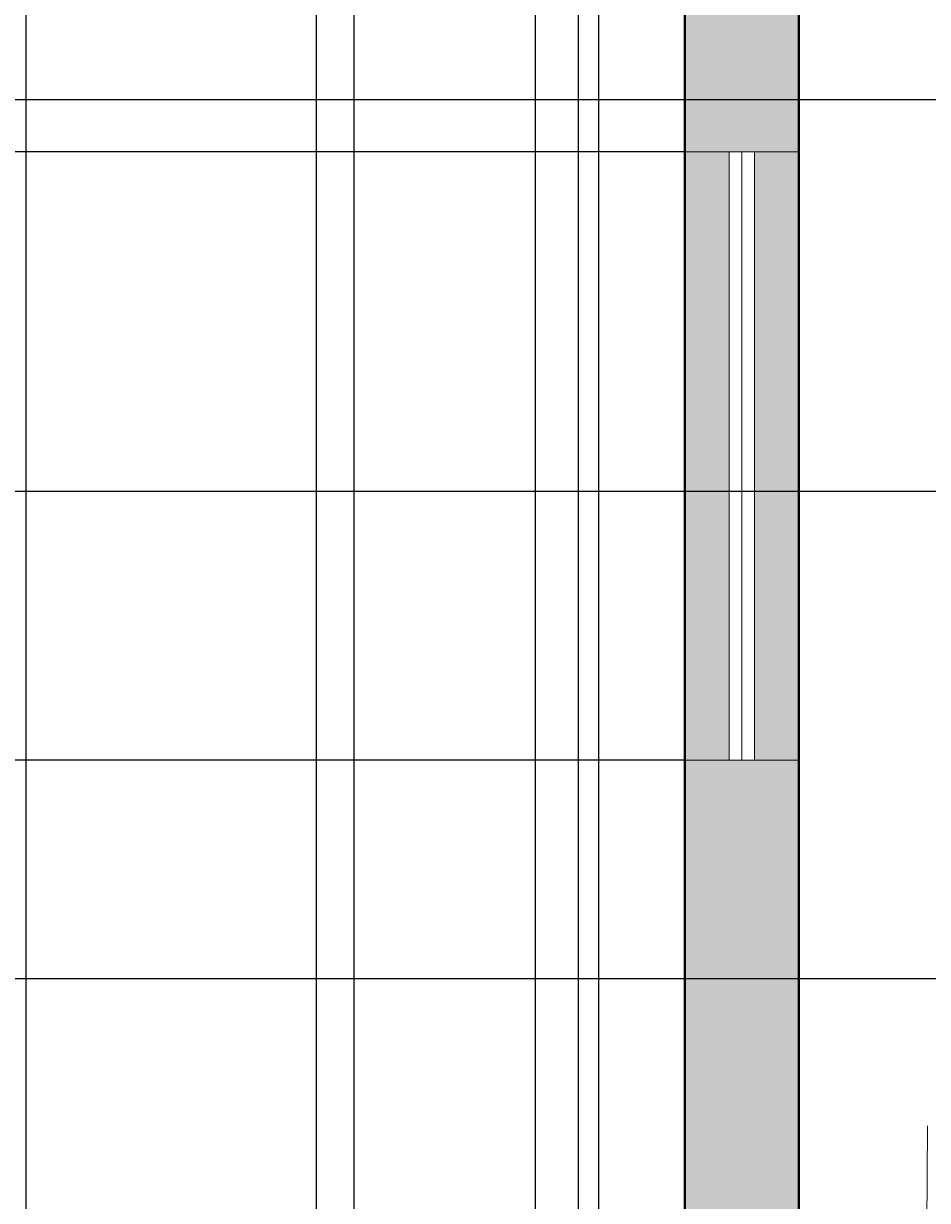
# Model space of a CAD drawing. Units: inches. Extents: x 818 to 1898, y 976 to 2364.
# Tile 33 of 96: x 1207 to 1278, y 1780 to 1873. Entities that reach past the tile are written whole.
import ezdxf

# ---------------------------------------------------------------- set-up
doc = ezdxf.new("R2010")
doc.units = ezdxf.units.IN
doc.header["$LTSCALE"] = 5
doc.header["$MEASUREMENT"] = 0
for name, color, linetype, lineweight in [('A-ANNO-DIMS', 2, 'Continuous', 18), ('A-FURN', 8, 'Continuous', 18), ('A-GLAZ', 4, 'Continuous', 18), ('A-WALL', 7, 'Continuous', 40)]:
    doc.layers.add(name, color=color, linetype=linetype, lineweight=lineweight)
doc.layers.add('A-GLAZ-PATT', color=141, linetype='Continuous', lineweight=9, true_color=0xadddf7)
doc.layers.add('A-WALL-PATT', color=251, linetype='Continuous', lineweight=13, true_color=0x636466)
doc.styles.get("Standard").update_dxf_attribs({"font": 'arial.ttf'})
doc.dimstyles.get("Standard").update_dxf_attribs({"dimtxt": 0.18, "dimasz": 0.18, "dimexe": 0.18, "dimexo": 0.0625, "dimgap": 0.09, "dimtad": 0, "dimtih": 1, "dimtoh": 1, "dimdec": 4, "dimzin": 0, "dimdsep": 46, "dimtxsty": 'Standard', "dimcen": 0.09, "dimadec": 0, "dimazin": 0, "dimtfac": 1, "dimtdec": 4, "dimtofl": 0, "dimtmove": 0, "dimatfit": 3, "dimfxl": 1, "dimtolj": 1, "dimtzin": 0, "dimarcsym": 0})

# ---------------------------------------------------------------- blocks, each defined once
blk = doc.blocks.new('SOFA-3-SEAT')
blk.add_line((74.051, 35.676), (39.879, 35.861))
blk = doc.blocks.new('*D59')
at = {"layer": 'A-ANNO-DIMS', "color": 0, "lineweight": -2, "ltscale": 5, "transparency": 16777216}
for p, q in [((1251.643, 2300.393), (818.026, 2300.393)), ((818.206, 2300.213), (818.206, 1669.95)), ((818.206, 1039.323), (818.206, 1669.586)), ((896.051, 1039.143), (818.026, 1039.143))]:
    blk.add_line(p, q, dxfattribs=at)
at = {"layer": 'A-ANNO-DIMS', "color": 0, "ltscale": 5, "transparency": 16777216}
for points in [[(818.176, 2300.213), (818.236, 2300.213), (818.206, 2300.393)], [(818.176, 1039.323), (818.236, 1039.323), (818.206, 1039.143)]]:
    blk.add_solid(points, dxfattribs=at)
at = {"layer": 'Defpoints', "color": 0, "ltscale": 5, "transparency": 16777216}
for p in [(818.206, 2300.393), (1251.706, 2300.393), (896.114, 1039.143)]:
    blk.add_point(p, dxfattribs=at)
at = {"layer": 'A-ANNO-DIMS', "color": 0, "ltscale": 5, "transparency": 16777216, "insert": (818.206, 1669.768), "char_height": 0.18, "attachment_point": 5}
blk.add_mtext('\\A1;1261.2', dxfattribs=at)
blk = doc.blocks.new('*D61')
at = {"layer": 'A-ANNO-DIMS', "color": 0, "lineweight": -2, "ltscale": 5, "transparency": 16777216}
for p, q in [((1071.725, 1203.027), (1071.725, 2363.873)), ((1071.905, 2363.693), (1250.936, 2363.693)), ((1430.545, 2363.693), (1251.514, 2363.693)), ((1430.725, 1203.027), (1430.725, 2363.873))]:
    blk.add_line(p, q, dxfattribs=at)
at = {"layer": 'A-ANNO-DIMS', "color": 0, "ltscale": 5, "transparency": 16777216}
for points in [[(1071.905, 2363.723), (1071.905, 2363.663), (1071.725, 2363.693)], [(1430.545, 2363.723), (1430.545, 2363.663), (1430.725, 2363.693)]]:
    blk.add_solid(points, dxfattribs=at)
at = {"layer": 'Defpoints', "color": 0, "ltscale": 5, "transparency": 16777216}
for p in [(1430.725, 2363.693), (1071.725, 1202.964), (1430.725, 1202.964)]:
    blk.add_point(p, dxfattribs=at)
at = {"layer": 'A-ANNO-DIMS', "color": 0, "ltscale": 5, "transparency": 16777216, "insert": (1251.225, 2363.693), "char_height": 0.18, "attachment_point": 5}
blk.add_mtext('\\A1;359', dxfattribs=at)
blk = doc.blocks.new('*D64')
at = {"layer": 'A-ANNO-DIMS', "color": 0, "lineweight": -2, "ltscale": 5, "transparency": 16777216}
for p, q in [((1197.725, 1501.141), (1197.725, 2363.873)), ((1197.905, 2363.693), (1313.935, 2363.693)), ((1430.545, 2363.693), (1314.516, 2363.693)), ((1430.725, 1501.141), (1430.725, 2363.873))]:
    blk.add_line(p, q, dxfattribs=at)
at = {"layer": 'A-ANNO-DIMS', "color": 0, "ltscale": 5, "transparency": 16777216}
for points in [[(1197.905, 2363.723), (1197.905, 2363.663), (1197.725, 2363.693)], [(1430.545, 2363.723), (1430.545, 2363.663), (1430.725, 2363.693)]]:
    blk.add_solid(points, dxfattribs=at)
at = {"layer": 'Defpoints', "color": 0, "ltscale": 5, "transparency": 16777216}
for p in [(1430.725, 2363.693), (1197.725, 1501.078), (1430.725, 1501.078)]:
    blk.add_point(p, dxfattribs=at)
at = {"layer": 'A-ANNO-DIMS', "color": 0, "ltscale": 5, "transparency": 16777216, "insert": (1314.225, 2363.693), "char_height": 0.18, "attachment_point": 5}
blk.add_mtext('\\A1;233', dxfattribs=at)
blk = doc.blocks.new('*D83')
at = {"layer": 'A-ANNO-DIMS', "color": 0, "lineweight": -2, "ltscale": 5, "transparency": 16777216}
for p, q in [((1197.725, 1700.141), (1197.725, 2363.873)), ((1197.905, 2363.693), (1228.023, 2363.693)), ((1258.545, 2363.693), (1228.427, 2363.693)), ((1258.725, 1700.141), (1258.725, 2363.873))]:
    blk.add_line(p, q, dxfattribs=at)
at = {"layer": 'A-ANNO-DIMS', "color": 0, "ltscale": 5, "transparency": 16777216}
for points in [[(1197.905, 2363.723), (1197.905, 2363.663), (1197.725, 2363.693)], [(1258.545, 2363.723), (1258.545, 2363.663), (1258.725, 2363.693)]]:
    blk.add_solid(points, dxfattribs=at)
at = {"layer": 'Defpoints', "color": 0, "ltscale": 5, "transparency": 16777216}
for p in [(1258.725, 2363.693), (1197.725, 1700.078), (1258.725, 1700.078)]:
    blk.add_point(p, dxfattribs=at)
at = {"layer": 'A-ANNO-DIMS', "color": 0, "ltscale": 5, "transparency": 16777216, "insert": (1228.225, 2363.693), "char_height": 0.18, "attachment_point": 5}
blk.add_mtext('\\A1;61', dxfattribs=at)
blk = doc.blocks.new('*D85')
at = {"layer": 'A-ANNO-DIMS', "color": 0, "lineweight": -2, "ltscale": 5, "transparency": 16777216}
for p, q in [((1258.788, 2053.078), (1897.916, 2053.078)), ((1897.736, 2052.898), (1897.736, 1876.76)), ((1897.736, 1700.258), (1897.736, 1876.396)), ((1258.788, 1700.078), (1897.916, 1700.078))]:
    blk.add_line(p, q, dxfattribs=at)
at = {"layer": 'A-ANNO-DIMS', "color": 0, "ltscale": 5, "transparency": 16777216}
for points in [[(1897.706, 2052.898), (1897.766, 2052.898), (1897.736, 2053.078)], [(1897.706, 1700.258), (1897.766, 1700.258), (1897.736, 1700.078)]]:
    blk.add_solid(points, dxfattribs=at)
at = {"layer": 'Defpoints', "color": 0, "ltscale": 5, "transparency": 16777216}
for p in [(1258.725, 2053.078), (1897.736, 2053.078), (1258.725, 1700.078)]:
    blk.add_point(p, dxfattribs=at)
at = {"layer": 'A-ANNO-DIMS', "color": 0, "ltscale": 5, "transparency": 16777216, "insert": (1897.736, 1876.578), "char_height": 0.18, "attachment_point": 5}
blk.add_mtext('\\A1;353', dxfattribs=at)
blk = doc.blocks.new('*D95')
at = {"layer": 'A-ANNO-DIMS', "color": 0, "lineweight": -2, "ltscale": 5, "transparency": 16777216}
for p, q in [((1173.542, 1071.118), (1173.542, 2363.873)), ((1173.722, 2363.693), (1201.288, 2363.693)), ((1229.467, 2363.693), (1201.901, 2363.693)), ((1229.647, 1071.118), (1229.647, 2363.873))]:
    blk.add_line(p, q, dxfattribs=at)
at = {"layer": 'A-ANNO-DIMS', "color": 0, "ltscale": 5, "transparency": 16777216}
for points in [[(1173.722, 2363.723), (1173.722, 2363.663), (1173.542, 2363.693)], [(1229.467, 2363.723), (1229.467, 2363.663), (1229.647, 2363.693)]]:
    blk.add_solid(points, dxfattribs=at)
at = {"layer": 'Defpoints', "color": 0, "ltscale": 5, "transparency": 16777216}
for p in [(1229.647, 2363.693), (1173.542, 1071.055), (1229.647, 1071.055)]:
    blk.add_point(p, dxfattribs=at)
at = {"layer": 'A-ANNO-DIMS', "color": 0, "ltscale": 5, "transparency": 16777216, "insert": (1201.595, 2363.693), "char_height": 0.18, "attachment_point": 5}
blk.add_mtext('\\A1;56.1', dxfattribs=at)
blk = doc.blocks.new('*D96')
at = {"layer": 'A-ANNO-DIMS', "color": 0, "lineweight": -2, "ltscale": 5, "transparency": 16777216}
for p, q in [((1229.647, 1071.118), (1229.647, 2363.873)), ((1229.827, 2363.693), (1256.516, 2363.693)), ((1283.99, 2363.693), (1257.301, 2363.693)), ((1284.17, 1071.118), (1284.17, 2363.873))]:
    blk.add_line(p, q, dxfattribs=at)
at = {"layer": 'A-ANNO-DIMS', "color": 0, "ltscale": 5, "transparency": 16777216}
for points in [[(1229.827, 2363.723), (1229.827, 2363.663), (1229.647, 2363.693)], [(1283.99, 2363.723), (1283.99, 2363.663), (1284.17, 2363.693)]]:
    blk.add_solid(points, dxfattribs=at)
at = {"layer": 'Defpoints', "color": 0, "ltscale": 5, "transparency": 16777216}
for p in [(1284.17, 2363.693), (1229.647, 1071.055), (1284.17, 1071.055)]:
    blk.add_point(p, dxfattribs=at)
at = {"layer": 'A-ANNO-DIMS', "color": 0, "ltscale": 5, "transparency": 16777216, "insert": (1256.909, 2363.693), "char_height": 0.18, "attachment_point": 5}
blk.add_mtext('\\A1;54.52', dxfattribs=at)
blk = doc.blocks.new('*D120')
at = {"layer": 'A-ANNO-DIMS', "color": 0, "lineweight": -2, "ltscale": 5, "transparency": 16777216}
for p, q in [((1766.29, 1797.717), (818.026, 1797.717)), ((818.206, 1797.537), (818.206, 1757.534)), ((818.206, 1717.167), (818.206, 1757.17)), ((1766.29, 1716.987), (818.026, 1716.987))]:
    blk.add_line(p, q, dxfattribs=at)
at = {"layer": 'A-ANNO-DIMS', "color": 0, "ltscale": 5, "transparency": 16777216}
for points in [[(818.176, 1797.537), (818.236, 1797.537), (818.206, 1797.717)], [(818.176, 1717.167), (818.236, 1717.167), (818.206, 1716.987)]]:
    blk.add_solid(points, dxfattribs=at)
at = {"layer": 'Defpoints', "color": 0, "ltscale": 5, "transparency": 16777216}
for p in [(818.206, 1797.717), (1766.352, 1797.717), (1766.352, 1716.987)]:
    blk.add_point(p, dxfattribs=at)
at = {"layer": 'A-ANNO-DIMS', "color": 0, "ltscale": 5, "transparency": 16777216, "insert": (818.206, 1757.352), "char_height": 0.18, "attachment_point": 5}
blk.add_mtext('\\A1;80.73', dxfattribs=at)
blk = doc.blocks.new('*D121')
at = {"layer": 'A-ANNO-DIMS', "color": 0, "lineweight": -2, "ltscale": 5, "transparency": 16777216}
for p, q in [((1766.29, 1884.203), (818.026, 1884.203)), ((818.206, 1884.023), (818.206, 1841.142)), ((818.206, 1797.897), (818.206, 1840.778)), ((1766.29, 1797.717), (818.026, 1797.717))]:
    blk.add_line(p, q, dxfattribs=at)
at = {"layer": 'A-ANNO-DIMS', "color": 0, "ltscale": 5, "transparency": 16777216}
for points in [[(818.176, 1884.023), (818.236, 1884.023), (818.206, 1884.203)], [(818.176, 1797.897), (818.236, 1797.897), (818.206, 1797.717)]]:
    blk.add_solid(points, dxfattribs=at)
at = {"layer": 'Defpoints', "color": 0, "ltscale": 5, "transparency": 16777216}
for p in [(818.206, 1884.203), (1766.352, 1884.203), (1766.352, 1797.717)]:
    blk.add_point(p, dxfattribs=at)
at = {"layer": 'A-ANNO-DIMS', "color": 0, "ltscale": 5, "transparency": 16777216, "insert": (818.206, 1840.96), "char_height": 0.18, "attachment_point": 5}
blk.add_mtext('\\A1;86.49', dxfattribs=at)
blk = doc.blocks.new('*D145')
at = {"layer": 'A-ANNO-DIMS', "color": 0, "lineweight": -2, "ltscale": 5, "transparency": 16777216}
for p, q in [((1197.393, 2122.314), (1197.393, 975.663)), ((1232.609, 2122.314), (1232.609, 975.663)), ((1197.573, 975.843), (1214.608, 975.843)), ((1232.429, 975.843), (1215.394, 975.843))]:
    blk.add_line(p, q, dxfattribs=at)
at = {"layer": 'A-ANNO-DIMS', "color": 0, "ltscale": 5, "transparency": 16777216}
for points in [[(1197.573, 975.873), (1197.573, 975.813), (1197.393, 975.843)], [(1232.429, 975.873), (1232.429, 975.813), (1232.609, 975.843)]]:
    blk.add_solid(points, dxfattribs=at)
at = {"layer": 'Defpoints', "color": 0, "ltscale": 5, "transparency": 16777216}
for p in [(1197.393, 2122.377), (1232.609, 2122.377), (1232.609, 975.843)]:
    blk.add_point(p, dxfattribs=at)
at = {"layer": 'A-ANNO-DIMS', "color": 0, "ltscale": 5, "transparency": 16777216, "insert": (1215.001, 975.843), "char_height": 0.18, "attachment_point": 5}
blk.add_mtext('\\A1;35.22', dxfattribs=at)
blk = doc.blocks.new('*D162')
at = {"layer": 'A-ANNO-DIMS', "color": 0, "lineweight": -2, "ltscale": 5, "transparency": 16777216}
for p, q in [((1429.163, 1876.078), (818.026, 1876.078)), ((818.206, 1875.898), (818.206, 1871.76)), ((818.206, 1867.258), (818.206, 1871.396)), ((1429.163, 1867.078), (818.026, 1867.078))]:
    blk.add_line(p, q, dxfattribs=at)
at = {"layer": 'A-ANNO-DIMS', "color": 0, "ltscale": 5, "transparency": 16777216}
for points in [[(818.176, 1875.898), (818.236, 1875.898), (818.206, 1876.078)], [(818.176, 1867.258), (818.236, 1867.258), (818.206, 1867.078)]]:
    blk.add_solid(points, dxfattribs=at)
at = {"layer": 'Defpoints', "color": 0, "ltscale": 5, "transparency": 16777216}
for p in [(1429.225, 1876.078), (818.206, 1867.078), (1429.225, 1867.078)]:
    blk.add_point(p, dxfattribs=at)
at = {"layer": 'A-ANNO-DIMS', "color": 0, "ltscale": 5, "transparency": 16777216, "insert": (818.206, 1871.578), "char_height": 0.18, "attachment_point": 5}
blk.add_mtext('\\A1;9', dxfattribs=at)
blk = doc.blocks.new('*D215')
at = {"layer": 'A-ANNO-DIMS', "color": 0, "lineweight": -2, "ltscale": 5, "transparency": 16777216}
for p, q in [((1590.663, 1876.078), (818.026, 1876.078)), ((818.206, 1875.898), (818.206, 1781.76)), ((818.206, 1687.258), (818.206, 1781.396)), ((1511.663, 1687.078), (818.026, 1687.078))]:
    blk.add_line(p, q, dxfattribs=at)
at = {"layer": 'A-ANNO-DIMS', "color": 0, "ltscale": 5, "transparency": 16777216}
for points in [[(818.176, 1875.898), (818.236, 1875.898), (818.206, 1876.078)], [(818.176, 1687.258), (818.236, 1687.258), (818.206, 1687.078)]]:
    blk.add_solid(points, dxfattribs=at)
at = {"layer": 'Defpoints', "color": 0, "ltscale": 5, "transparency": 16777216}
for p in [(818.206, 1876.078), (1590.725, 1876.078), (1511.725, 1687.078)]:
    blk.add_point(p, dxfattribs=at)
at = {"layer": 'A-ANNO-DIMS', "color": 0, "ltscale": 5, "transparency": 16777216, "insert": (818.206, 1781.578), "char_height": 0.18, "attachment_point": 5}
blk.add_mtext('\\A1;189', dxfattribs=at)
blk = doc.blocks.new('*D227')
at = {"layer": 'A-ANNO-DIMS', "color": 0, "lineweight": -2, "ltscale": 5, "transparency": 16777216}
for p, q in [((1595.663, 1867.078), (818.026, 1867.078)), ((818.206, 1866.898), (818.206, 1851.813)), ((818.206, 1836.364), (818.206, 1851.449)), ((1594.663, 1836.184), (818.026, 1836.184))]:
    blk.add_line(p, q, dxfattribs=at)
at = {"layer": 'A-ANNO-DIMS', "color": 0, "ltscale": 5, "transparency": 16777216}
for points in [[(818.176, 1866.898), (818.236, 1866.898), (818.206, 1867.078)], [(818.176, 1836.364), (818.236, 1836.364), (818.206, 1836.184)]]:
    blk.add_solid(points, dxfattribs=at)
at = {"layer": 'Defpoints', "color": 0, "ltscale": 5, "transparency": 16777216}
for p in [(818.206, 1867.078), (1595.725, 1867.078), (1594.725, 1836.184)]:
    blk.add_point(p, dxfattribs=at)
at = {"layer": 'A-ANNO-DIMS', "color": 0, "ltscale": 5, "transparency": 16777216, "insert": (818.206, 1851.631), "char_height": 0.18, "attachment_point": 5}
blk.add_mtext('\\A1;30.894', dxfattribs=at)
blk = doc.blocks.new('*D233')
at = {"layer": 'A-ANNO-DIMS', "color": 0, "lineweight": -2, "ltscale": 5, "transparency": 16777216}
for p, q in [((1267.725, 2044.016), (1267.725, 975.663)), ((1303.931, 2008.329), (1303.931, 975.663)), ((1267.905, 975.843), (1285.365, 975.843)), ((1303.751, 975.843), (1286.292, 975.843))]:
    blk.add_line(p, q, dxfattribs=at)
at = {"layer": 'A-ANNO-DIMS', "color": 0, "ltscale": 5, "transparency": 16777216}
for points in [[(1267.905, 975.873), (1267.905, 975.813), (1267.725, 975.843)], [(1303.751, 975.873), (1303.751, 975.813), (1303.931, 975.843)]]:
    blk.add_solid(points, dxfattribs=at)
at = {"layer": 'Defpoints', "color": 0, "ltscale": 5, "transparency": 16777216}
for p in [(1267.725, 2044.078), (1303.931, 2008.392), (1303.931, 975.843)]:
    blk.add_point(p, dxfattribs=at)
at = {"layer": 'A-ANNO-DIMS', "color": 0, "ltscale": 5, "transparency": 16777216, "insert": (1285.828, 975.843), "char_height": 0.18, "attachment_point": 5}
blk.add_mtext('\\A1;36.206', dxfattribs=at)
blk = doc.blocks.new('*D247')
at = {"layer": 'A-ANNO-DIMS', "color": 0, "lineweight": -2, "ltscale": 5, "transparency": 16777216}
for p, q in [((1258.663, 1862.965), (818.026, 1862.965)), ((818.206, 1862.785), (818.206, 1839.147)), ((818.206, 1815.145), (818.206, 1838.783)), ((1258.663, 1814.965), (818.026, 1814.965))]:
    blk.add_line(p, q, dxfattribs=at)
at = {"layer": 'A-ANNO-DIMS', "color": 0, "ltscale": 5, "transparency": 16777216}
for points in [[(818.176, 1862.785), (818.236, 1862.785), (818.206, 1862.965)], [(818.176, 1815.145), (818.236, 1815.145), (818.206, 1814.965)]]:
    blk.add_solid(points, dxfattribs=at)
at = {"layer": 'Defpoints', "color": 0, "ltscale": 5, "transparency": 16777216}
for p in [(818.206, 1862.965), (1258.725, 1862.965), (1258.725, 1814.965)]:
    blk.add_point(p, dxfattribs=at)
at = {"layer": 'A-ANNO-DIMS', "color": 0, "ltscale": 5, "transparency": 16777216, "insert": (818.206, 1838.965), "char_height": 0.18, "attachment_point": 5}
blk.add_mtext('\\A1;48', dxfattribs=at)
blk = doc.blocks.new('*D249')
at = {"layer": 'A-ANNO-DIMS', "color": 0, "lineweight": -2, "ltscale": 5, "transparency": 16777216}
for p, q in [((1258.663, 1814.965), (818.026, 1814.965)), ((818.206, 1814.785), (818.206, 1785.331)), ((818.206, 1755.512), (818.206, 1784.967)), ((1258.663, 1755.332), (818.026, 1755.332))]:
    blk.add_line(p, q, dxfattribs=at)
at = {"layer": 'A-ANNO-DIMS', "color": 0, "ltscale": 5, "transparency": 16777216}
for points in [[(818.176, 1814.785), (818.236, 1814.785), (818.206, 1814.965)], [(818.176, 1755.512), (818.236, 1755.512), (818.206, 1755.332)]]:
    blk.add_solid(points, dxfattribs=at)
at = {"layer": 'Defpoints', "color": 0, "ltscale": 5, "transparency": 16777216}
for p in [(818.206, 1814.965), (1258.725, 1814.965), (1258.725, 1755.332)]:
    blk.add_point(p, dxfattribs=at)
at = {"layer": 'A-ANNO-DIMS', "color": 0, "ltscale": 5, "transparency": 16777216, "insert": (818.206, 1785.149), "char_height": 0.18, "attachment_point": 5}
blk.add_mtext('\\A1;59.63', dxfattribs=at)
blk = doc.blocks.new('*D251')
at = {"layer": 'A-ANNO-DIMS', "color": 0, "lineweight": -2, "ltscale": 5, "transparency": 16777216}
for p, q in [((1250.303, 1878.329), (1250.303, 975.663)), ((1258.725, 1878.329), (1258.725, 975.663)), ((1250.483, 975.843), (1254.121, 975.843)), ((1258.545, 975.843), (1254.907, 975.843))]:
    blk.add_line(p, q, dxfattribs=at)
at = {"layer": 'A-ANNO-DIMS', "color": 0, "ltscale": 5, "transparency": 16777216}
for points in [[(1250.483, 975.873), (1250.483, 975.813), (1250.303, 975.843)], [(1258.545, 975.873), (1258.545, 975.813), (1258.725, 975.843)]]:
    blk.add_solid(points, dxfattribs=at)
at = {"layer": 'Defpoints', "color": 0, "ltscale": 5, "transparency": 16777216}
for p in [(1250.303, 1878.392), (1258.725, 1878.392), (1258.725, 975.843)]:
    blk.add_point(p, dxfattribs=at)
at = {"layer": 'A-ANNO-DIMS', "color": 0, "ltscale": 5, "transparency": 16777216, "insert": (1254.514, 975.843), "char_height": 0.18, "attachment_point": 5}
blk.add_mtext('\\A1;8.422', dxfattribs=at)
blk = doc.blocks.new('*D254')
at = {"layer": 'A-ANNO-DIMS', "color": 0, "lineweight": -2, "ltscale": 5, "transparency": 16777216}
for p, q in [((1267.725, 2044.016), (1267.725, 975.663)), ((1330.305, 2044.016), (1330.305, 975.663)), ((1267.905, 975.843), (1298.621, 975.843)), ((1330.125, 975.843), (1299.409, 975.843))]:
    blk.add_line(p, q, dxfattribs=at)
at = {"layer": 'A-ANNO-DIMS', "color": 0, "ltscale": 5, "transparency": 16777216}
for points in [[(1267.905, 975.873), (1267.905, 975.813), (1267.725, 975.843)], [(1330.125, 975.873), (1330.125, 975.813), (1330.305, 975.843)]]:
    blk.add_solid(points, dxfattribs=at)
at = {"layer": 'Defpoints', "color": 0, "ltscale": 5, "transparency": 16777216}
for p in [(1267.725, 2044.078), (1330.305, 2044.078), (1330.305, 975.843)]:
    blk.add_point(p, dxfattribs=at)
at = {"layer": 'A-ANNO-DIMS', "color": 0, "ltscale": 5, "transparency": 16777216, "insert": (1299.015, 975.843), "char_height": 0.18, "attachment_point": 5}
blk.add_mtext('\\A1;62.58', dxfattribs=at)
blk = doc.blocks.new('*D269')
at = {"layer": 'A-ANNO-DIMS', "color": 0, "lineweight": -2, "ltscale": 5, "transparency": 16777216}
for p, q in [((1246.938, 1534.141), (1246.938, 2363.873)), ((1247.118, 2363.693), (1293.706, 2363.693)), ((1341.079, 2363.693), (1294.491, 2363.693)), ((1341.259, 1534.141), (1341.259, 2363.873))]:
    blk.add_line(p, q, dxfattribs=at)
at = {"layer": 'A-ANNO-DIMS', "color": 0, "ltscale": 5, "transparency": 16777216}
for points in [[(1247.118, 2363.723), (1247.118, 2363.663), (1246.938, 2363.693)], [(1341.079, 2363.723), (1341.079, 2363.663), (1341.259, 2363.693)]]:
    blk.add_solid(points, dxfattribs=at)
at = {"layer": 'Defpoints', "color": 0, "ltscale": 5, "transparency": 16777216}
for p in [(1341.259, 2363.693), (1246.938, 1534.078), (1341.259, 1534.078)]:
    blk.add_point(p, dxfattribs=at)
at = {"layer": 'A-ANNO-DIMS', "color": 0, "ltscale": 5, "transparency": 16777216, "insert": (1294.099, 2363.693), "char_height": 0.18, "attachment_point": 5}
blk.add_mtext('\\A1;94.32', dxfattribs=at)
blk = doc.blocks.new('*D271')
at = {"layer": 'A-ANNO-DIMS', "color": 0, "lineweight": -2, "ltscale": 5, "transparency": 16777216}
for p, q in [((1206.725, 1510.141), (1206.725, 2363.873)), ((1206.905, 2363.693), (1226.451, 2363.693)), ((1246.758, 2363.693), (1227.211, 2363.693)), ((1246.938, 1510.141), (1246.938, 2363.873))]:
    blk.add_line(p, q, dxfattribs=at)
at = {"layer": 'A-ANNO-DIMS', "color": 0, "ltscale": 5, "transparency": 16777216}
for points in [[(1206.905, 2363.723), (1206.905, 2363.663), (1206.725, 2363.693)], [(1246.758, 2363.723), (1246.758, 2363.663), (1246.938, 2363.693)]]:
    blk.add_solid(points, dxfattribs=at)
at = {"layer": 'Defpoints', "color": 0, "ltscale": 5, "transparency": 16777216}
for p in [(1246.938, 2363.693), (1206.725, 1510.078), (1246.938, 1510.078)]:
    blk.add_point(p, dxfattribs=at)
at = {"layer": 'A-ANNO-DIMS', "color": 0, "ltscale": 5, "transparency": 16777216, "insert": (1226.831, 2363.693), "char_height": 0.18, "attachment_point": 5}
blk.add_mtext('\\A1;40.21', dxfattribs=at)
blk = doc.blocks.new('*D276')
at = {"layer": 'A-ANNO-DIMS', "color": 0, "lineweight": -2, "ltscale": 5, "transparency": 16777216}
for p, q in [((1206.725, 1687.141), (1206.725, 2363.873)), ((1206.905, 2363.693), (1228.949, 2363.693)), ((1251.753, 2363.693), (1229.709, 2363.693)), ((1251.933, 1681.439), (1251.933, 2363.873))]:
    blk.add_line(p, q, dxfattribs=at)
at = {"layer": 'A-ANNO-DIMS', "color": 0, "ltscale": 5, "transparency": 16777216}
for points in [[(1206.905, 2363.723), (1206.905, 2363.663), (1206.725, 2363.693)], [(1251.753, 2363.723), (1251.753, 2363.663), (1251.933, 2363.693)]]:
    blk.add_solid(points, dxfattribs=at)
at = {"layer": 'Defpoints', "color": 0, "ltscale": 5, "transparency": 16777216}
for p in [(1251.933, 2363.693), (1206.725, 1687.078), (1251.933, 1681.376)]:
    blk.add_point(p, dxfattribs=at)
at = {"layer": 'A-ANNO-DIMS', "color": 0, "ltscale": 5, "transparency": 16777216, "insert": (1229.329, 2363.693), "char_height": 0.18, "attachment_point": 5}
blk.add_mtext('\\A1;45.21', dxfattribs=at)
blk = doc.blocks.new('*D285')
at = {"layer": 'A-ANNO-DIMS', "color": 0, "lineweight": -2, "ltscale": 5, "transparency": 16777216}
for p, q in [((1305.828, 1830.022), (1305.828, 975.663)), ((1267.725, 1814.903), (1267.725, 975.663)), ((1267.905, 975.843), (1286.47, 975.843)), ((1305.648, 975.843), (1287.083, 975.843))]:
    blk.add_line(p, q, dxfattribs=at)
at = {"layer": 'A-ANNO-DIMS', "color": 0, "ltscale": 5, "transparency": 16777216}
for points in [[(1267.905, 975.873), (1267.905, 975.813), (1267.725, 975.843)], [(1305.648, 975.873), (1305.648, 975.813), (1305.828, 975.843)]]:
    blk.add_solid(points, dxfattribs=at)
at = {"layer": 'Defpoints', "color": 0, "ltscale": 5, "transparency": 16777216}
for p in [(1305.828, 1830.084), (1267.725, 1814.965), (1267.725, 975.843)]:
    blk.add_point(p, dxfattribs=at)
at = {"layer": 'A-ANNO-DIMS', "color": 0, "ltscale": 5, "transparency": 16777216, "insert": (1286.776, 975.843), "char_height": 0.18, "attachment_point": 5}
blk.add_mtext('\\A1;38.1', dxfattribs=at)

msp = doc.modelspace()

# ---------------------------------------------------------------- hatches: boundary and pattern name
at = {"layer": 'A-GLAZ-PATT', "ltscale": 5}
h = msp.add_hatch(color=256, dxfattribs=at)
h.dxf.hatch_style = 1
h.paths.add_polyline_path([(1283.8183, 1504.5782), (1206.7251, 1504.5782), (1206.7251, 1501.0782), (1283.8183, 1501.0782)])
h.paths.add_polyline_path([(1283.8183, 1510.0782), (1206.7251, 1510.0782), (1206.7251, 1506.5782), (1283.8183, 1506.5782)])
h.paths.add_polyline_path([(1490.9163, 1355.0782), (1439.7252, 1355.0782), (1439.7252, 1409.0522), (1436.2252, 1409.0522), (1436.2252, 1351.5782), (1490.9163, 1351.5782)])
h.paths.add_polyline_path([(1434.2252, 1409.0522), (1430.7251, 1409.0522), (1430.7251, 1346.0782), (1435.0799, 1346.0782), (1435.0731, 1346.1152), (1435.1501, 1346.0782), (1490.9163, 1346.0782), (1490.9163, 1349.5782), (1434.2252, 1349.5782)])
h.paths.add_polyline_path([(1714.7252, 1545.0782), (1711.2252, 1545.0782), (1711.2252, 1521.0782), (1714.7252, 1521.0782)])
h.paths.add_polyline_path([(1709.2252, 1545.0782), (1705.7252, 1545.0782), (1705.7252, 1521.0782), (1709.2252, 1521.0782)])
h.paths.add_polyline_path([(1714.7252, 1687.0782), (1711.2252, 1687.0782), (1711.2252, 1649.9029), (1714.7252, 1649.9029)])
h.paths.add_polyline_path([(1709.2252, 1687.0782), (1705.7252, 1687.0782), (1705.7252, 1649.9029), (1709.2252, 1649.9029)])
h.paths.add_polyline_path([(1709.2252, 1745.5584), (1705.7252, 1745.5584), (1705.7252, 1717.3178), (1709.2252, 1717.3178)])
h.paths.add_polyline_path([(1714.7252, 1745.5584), (1711.2252, 1745.5584), (1711.2252, 1717.3178), (1714.7252, 1717.3178)])
h.paths.add_polyline_path([(1714.7252, 2014.5114), (1711.2252, 2014.5114), (1711.2252, 1962.0338), (1714.7252, 1962.0338)])
h.paths.add_polyline_path([(1709.2252, 2014.5114), (1705.7252, 2014.5114), (1705.7252, 1962.0338), (1709.2252, 1962.0338)])
h.paths.add_polyline_path([(1538.5155, 2047.5782), (1485.1216, 2047.5782), (1485.1216, 2044.0782), (1538.5155, 2044.0782)])
h.paths.add_polyline_path([(1538.5155, 2053.0782), (1485.1216, 2053.0782), (1485.1216, 2049.5782), (1538.5155, 2049.5782)])
h.paths.add_polyline_path([(1388.0315, 2047.5782), (1330.305, 2047.5782), (1330.305, 2044.0782), (1388.0315, 2044.0782)])
h.paths.add_polyline_path([(1388.0315, 2053.0782), (1330.305, 2053.0782), (1330.305, 2049.5782), (1388.0315, 2049.5782)])
h.paths.add_polyline_path([(1262.2252, 2019.2871), (1258.7251, 2019.2871), (1258.7251, 1928.9218), (1262.2252, 1928.9218)])
h.paths.add_polyline_path([(1267.7251, 2019.2871), (1264.2252, 2019.2871), (1264.2252, 1928.9218), (1267.7251, 1928.9218)])
h.paths.add_polyline_path([(1262.2252, 1862.9652), (1258.7251, 1862.9652), (1258.7251, 1814.9652), (1262.2252, 1814.9652)])
h.paths.add_polyline_path([(1267.7251, 1862.9652), (1264.2252, 1862.9652), (1264.2252, 1814.9652), (1267.7251, 1814.9652)])
h.paths.add_polyline_path([(1262.2252, 1755.3321), (1258.7251, 1755.3321), (1258.7251, 1707.3321), (1262.2252, 1707.3321)])
h.paths.add_polyline_path([(1267.7251, 1755.3321), (1264.2252, 1755.3321), (1264.2252, 1707.3321), (1267.7251, 1707.3321)])
h.paths.add_polyline_path([(1251.9333, 1692.5782), (1206.7251, 1692.5782), (1206.7251, 1687.0782), (1251.9333, 1687.0782)])
h.paths.add_polyline_path([(1251.9333, 1700.0782), (1206.7251, 1700.0782), (1206.7251, 1694.5782), (1251.9333, 1694.5782)])
at = {"layer": 'A-WALL-PATT', "ltscale": 5}
h = msp.add_hatch(color=256, dxfattribs=at)
h.dxf.hatch_style = 1
h.paths.add_polyline_path([(1267.7251, 1928.9218), (1258.7251, 1928.9218), (1258.7251, 1913.6401), (1250.3029, 1913.6401), (1250.3029, 1878.3919), (1258.7251, 1878.3919), (1258.7251, 1862.9652), (1267.7251, 1862.9652)])
h.paths.add_polyline_path([(1267.7251, 1814.9652), (1258.7251, 1814.9652), (1258.7251, 1755.3321), (1267.7251, 1755.3321)])
h.paths.add_polyline_path([(1463.7252, 1696.0782), (1267.7251, 1696.0782), (1267.7251, 1707.3321), (1258.7251, 1707.3321), (1258.7251, 1700.0782), (1251.9333, 1700.0782), (1251.9333, 1687.0782), (1463.7252, 1687.0782)])
h.paths.add_polyline_path([(1714.7252, 1717.3178), (1705.7252, 1717.3178), (1705.7252, 1696.0782), (1599.7252, 1696.0782), (1599.7252, 1790.0782), (1705.7252, 1790.0782), (1705.7252, 1785.6125), (1714.7252, 1785.6125), (1714.7252, 1827.2125), (1705.7252, 1827.2125), (1705.7252, 1802.0782), (1599.7252, 1802.0782), (1599.7252, 1867.0782), (1705.7252, 1867.0782), (1705.7252, 1857.2125), (1714.7252, 1857.2125), (1714.7252, 1930.0316), (1741.8409, 1930.0316), (1741.8409, 1935.0316), (1714.7252, 1935.0316), (1714.7252, 1957.0338), (1741.8409, 1957.0338), (1741.8409, 1962.0338), (1714.7252, 1962.0338), (1705.7252, 1962.0338), (1705.7252, 1948.0782), (1599.7252, 1948.0782), (1599.7252, 1981.0782), (1590.7251, 1981.0782), (1590.7251, 1941.0782), (1620.7252, 1941.0782), (1705.7252, 1941.0782), (1705.7252, 1876.0782), (1599.7252, 1876.0782), (1599.7252, 1911.0782), (1590.7251, 1911.0782), (1590.7251, 1876.0782), (1429.2251, 1876.0782), (1429.2251, 1867.0782), (1511.7251, 1867.0782), (1528.593, 1867.0782), (1595.7251, 1867.0782), (1595.7251, 1773.0782), (1520.7252, 1773.0782), (1520.7252, 1837.5823), (1532.593, 1837.5823), (1532.593, 1867.0782), (1528.593, 1867.0782), (1528.593, 1841.5823), (1511.7251, 1841.5823), (1511.7251, 1744.9714), (1520.7252, 1744.9714), (1520.7252, 1761.0782), (1595.7251, 1761.0782), (1595.7251, 1696.0782), (1520.7252, 1696.0782), (1520.7252, 1716.0454), (1511.7251, 1716.0454), (1511.7251, 1696.0782), (1511.7251, 1687.0782), (1714.7252, 1687.0782)])
h.paths.add_polyline_path([(1714.7252, 2053.0782), (1714.7252, 2081.1881), (1709.7252, 2081.1881), (1709.7252, 2053.0782), (1681.6446, 2053.0782), (1681.6446, 2081.1881), (1676.6446, 2081.1881), (1676.6446, 2053.0782), (1538.5155, 2053.0782), (1538.5155, 2044.0782), (1590.7251, 2044.0782), (1590.7251, 2011.0782), (1599.7252, 2011.0782), (1599.7252, 2044.0782), (1705.7252, 2044.0782), (1705.7252, 2014.5114), (1714.7252, 2014.5114)])
h.paths.add_polyline_path([(1485.1216, 2053.0782), (1422.02, 2053.0782), (1422.02, 2081.1881), (1413.02, 2081.1881), (1413.02, 2053.0782), (1399.6356, 2053.0782), (1399.6356, 2081.1881), (1390.6356, 2081.1881), (1390.6356, 2053.0782), (1388.0315, 2053.0782), (1388.0315, 2044.0782), (1416.2743, 2044.0782), (1485.1216, 2044.0782)])
h.paths.add_polyline_path([(1330.305, 2053.0782), (1258.7251, 2053.0782), (1258.7251, 2019.2871), (1267.7251, 2019.2871), (1267.7251, 2044.0782), (1330.305, 2044.0782)])
h.paths.add_polyline_path([(1258.7251, 2053.0782), (1214.6577, 2053.0782), (1214.6577, 2044.0782), (1258.7251, 2044.0782)])
h.paths.add_polyline_path([(1214.6577, 2053.0782), (1180.349, 2053.0782), (1180.349, 2044.0782), (1214.6577, 2044.0782)])
h.paths.add_polyline_path([(1714.7252, 1639.5782), (1741.8409, 1639.5782), (1741.8409, 1643.5782), (1714.7252, 1643.5782), (1714.7252, 1649.9029), (1705.7252, 1649.9029), (1705.7252, 1600.0782), (1477.7252, 1600.0782), (1477.7252, 1591.0782), (1520.7252, 1591.0782), (1616.7252, 1591.0782), (1616.7252, 1416.6857), (1622.7252, 1416.6857), (1622.7252, 1463.0782), (1624.7252, 1463.0782), (1624.7252, 1467.0782), (1622.7252, 1467.0782), (1622.7252, 1591.0782), (1705.7252, 1591.0782), (1705.7252, 1545.0782), (1714.7252, 1545.0782), (1741.8409, 1545.0782), (1741.8409, 1549.0782), (1714.7252, 1549.0782), (1714.7252, 1593.9175), (1737.8409, 1593.9175), (1737.8409, 1597.9175), (1714.7252, 1597.9175)])
h.paths.add_polyline_path([(1674.9024, 2060.7419), (1714.7045, 2060.7419), (1714.7045, 2073.1061), (1674.9024, 2073.1061)], flags=25)
h.paths.add_polyline_path([(1394.5468, 2061.6618), (1422.2344, 2061.6618), (1422.2344, 2074.0261), (1394.5468, 2074.0261)], flags=24)

# ---------------------------------------------------------------- linework, layer by layer
at = {"layer": 'A-GLAZ'}
for p, q in [((1267.7251, 1862.9652), (1258.7251, 1862.9652)), ((1262.2252, 1862.9652), (1262.2252, 1814.9652)), ((1263.2252, 1862.9652), (1263.2252, 1814.9652)), ((1264.2252, 1862.9652), (1264.2252, 1814.9652)), ((1267.7251, 1814.9652), (1258.7251, 1814.9652))]:
    msp.add_line(p, q, dxfattribs=at)
at = {"layer": 'A-WALL'}
for p, q in [((1267.7251, 2044.0782), (1267.7251, 1862.9652)), ((1258.7251, 1878.3919), (1258.7251, 1700.0782)), ((1267.7251, 1867.0782), (1267.7251, 1696.0782))]:
    msp.add_line(p, q, dxfattribs=at)

# ---------------------------------------------------------------- block references
at = {"layer": 'A-FURN', "rotation": 90.0000000000007}
msp.add_blockref('SOFA-3-SEAT', (1313.5566, 1712.0791), dxfattribs=at)

# ---------------------------------------------------------------- dimensions: what is measured, and where the dimension line sits
at = {"layer": 'A-ANNO-DIMS', "ltscale": 5}
for base, p1, p2, override, picture, middle in [((1430.7251, 2363.6929), (1071.7251, 1202.9642), (1430.7251, 1202.9642), {"dimdec": 0, "dimlfac": 1, "dimrnd": 0, "dimzin": 0, "dimdsep": 46, "dimlunit": 2}, '*D61', (1251.2251, 2363.6929)), ((1229.6474, 2363.6929), (1173.5418, 1071.0552), (1229.6474, 1071.0552), {"dimdec": 1, "dimlfac": 1, "dimrnd": 0, "dimzin": 0, "dimdsep": 46, "dimlunit": 2}, '*D95', (1201.5946, 2363.6929)), ((1430.7251, 2363.6929), (1197.7251, 1501.0782), (1430.7251, 1501.0782), {"dimdec": 0, "dimlfac": 1, "dimrnd": 0, "dimzin": 0, "dimdsep": 46, "dimlunit": 2}, '*D64', (1314.2251, 2363.6929)), ((1258.7251, 2363.6929), (1197.7251, 1700.0782), (1258.7251, 1700.0782), {"dimdec": 0, "dimlfac": 1, "dimrnd": 0, "dimzin": 0, "dimdsep": 46, "dimlunit": 2}, '*D83', (1228.2251, 2363.6929)), ((1246.9377, 2363.6929), (1206.7251, 1510.0782), (1246.9377, 1510.0782), {"dimdec": 2, "dimlfac": 1, "dimrnd": 0, "dimzin": 0, "dimdsep": 46, "dimlunit": 2}, '*D271', (1226.8314, 2363.6929)), ((1251.9333, 2363.6929), (1206.7251, 1687.0782), (1251.9333, 1681.3763), {"dimdec": 2, "dimlfac": 1, "dimrnd": 0, "dimzin": 0, "dimdsep": 46, "dimlunit": 2}, '*D276', (1229.3292, 2363.6929)), ((1284.1697, 2363.6929), (1229.6474, 1071.0552), (1284.1697, 1071.0552), {"dimdec": 2, "dimlfac": 1, "dimrnd": 0, "dimzin": 0, "dimdsep": 46, "dimlunit": 2}, '*D96', (1256.9085, 2363.6929)), ((1341.2593, 2363.6929), (1246.9377, 1534.0782), (1341.2593, 1534.0782), {"dimdec": 2, "dimlfac": 1, "dimrnd": 0, "dimzin": 0, "dimdsep": 46, "dimlunit": 2}, '*D269', (1294.0985, 2363.6929)), ((1232.6091, 975.8433), (1197.3925, 2122.3767), (1232.6091, 2122.3767), {"dimdec": 2, "dimlfac": 1, "dimrnd": 0, "dimzin": 0, "dimdsep": 46, "dimlunit": 2}, '*D145', (1215.0008, 975.8433)), ((1303.9314, 975.8433), (1267.7251, 2044.0782), (1303.9314, 2008.3917), {"dimdec": 3, "dimlfac": 1, "dimrnd": 0, "dimzin": 0, "dimdsep": 46, "dimlunit": 2}, '*D233', (1285.8283, 975.8433)), ((1330.305, 975.8433), (1267.7251, 2044.0782), (1330.305, 2044.0782), {"dimdec": 2, "dimlfac": 1, "dimrnd": 0, "dimzin": 0, "dimdsep": 46, "dimlunit": 2}, '*D254', (1299.0151, 975.8433)), ((1258.7251, 975.8433), (1250.3029, 1878.3919), (1258.7251, 1878.3919), {"dimdec": 3, "dimlfac": 1, "dimrnd": 0, "dimzin": 0, "dimdsep": 46, "dimlunit": 2}, '*D251', (1254.514, 975.8433)), ((1267.7251, 975.8433), (1305.8278, 1830.0844), (1267.7251, 1814.9652), {"dimdec": 1, "dimlfac": 1, "dimrnd": 0, "dimzin": 0, "dimdsep": 46, "dimlunit": 2}, '*D285', (1286.7765, 975.8433))]:
    dim = msp.add_linear_dim(base=base, p1=p1, p2=p2, dimstyle='Standard', override=override, dxfattribs=at)
    dim.commit()
    dim.dimension.update_dxf_attribs({"geometry": picture, "text_midpoint": middle})
for base, p1, p2, override, picture, middle in [((818.2059, 2300.3929), (896.1138, 1039.1433), (1251.7057, 2300.3929), {"dimdec": 1, "dimlfac": 1, "dimrnd": 0, "dimzin": 0, "dimdsep": 46, "dimlunit": 2}, '*D59', (818.2059, 1669.7681)), ((1897.736, 2053.0782), (1258.7251, 1700.0782), (1258.7251, 2053.0782), {"dimdec": 0, "dimlfac": 1, "dimrnd": 0, "dimzin": 0, "dimdsep": 46, "dimlunit": 2}, '*D85', (1897.736, 1876.5782)), ((818.2059, 1884.2031), (1766.3524, 1797.7165), (1766.3524, 1884.2031), {"dimdec": 2, "dimlfac": 1, "dimrnd": 0, "dimzin": 0, "dimdsep": 46, "dimlunit": 2}, '*D121', (818.2059, 1840.9598)), ((818.2059, 1876.0782), (1511.7251, 1687.0782), (1590.7251, 1876.0782), {"dimdec": 0, "dimlfac": 1, "dimrnd": 0, "dimzin": 0, "dimdsep": 46, "dimlunit": 2}, '*D215', (818.2059, 1781.5782)), ((818.2059, 1867.0782), (1429.2251, 1876.0782), (1429.2251, 1867.0782), {"dimdec": 0, "dimlfac": 1, "dimrnd": 0, "dimzin": 0, "dimdsep": 46, "dimlunit": 2}, '*D162', (818.2059, 1871.5782)), ((818.2059, 1867.0782), (1594.7251, 1836.1844), (1595.7251, 1867.0782), {"dimdec": 3, "dimlfac": 1, "dimrnd": 0, "dimzin": 0, "dimdsep": 46, "dimlunit": 2}, '*D227', (818.2059, 1851.6313)), ((818.2059, 1862.9652), (1258.7251, 1814.9652), (1258.7251, 1862.9652), {"dimdec": 0, "dimlfac": 1, "dimrnd": 0, "dimzin": 0, "dimdsep": 46, "dimlunit": 2}, '*D247', (818.2059, 1838.9652)), ((818.2059, 1814.9652), (1258.7251, 1755.3321), (1258.7251, 1814.9652), {"dimdec": 2, "dimlfac": 1, "dimrnd": 0, "dimzin": 0, "dimdsep": 46, "dimlunit": 2}, '*D249', (818.2059, 1785.1486)), ((818.2059, 1797.7165), (1766.3524, 1716.9866), (1766.3524, 1797.7165), {"dimdec": 2, "dimlfac": 1, "dimrnd": 0, "dimzin": 0, "dimdsep": 46, "dimlunit": 2}, '*D120', (818.2059, 1757.3516))]:
    dim = msp.add_linear_dim(base=base, p1=p1, p2=p2, angle=90, dimstyle='Standard', override=override, dxfattribs=at)
    dim.commit()
    dim.dimension.update_dxf_attribs({"geometry": picture, "text_midpoint": middle})

doc.saveas('drawing.dxf')
